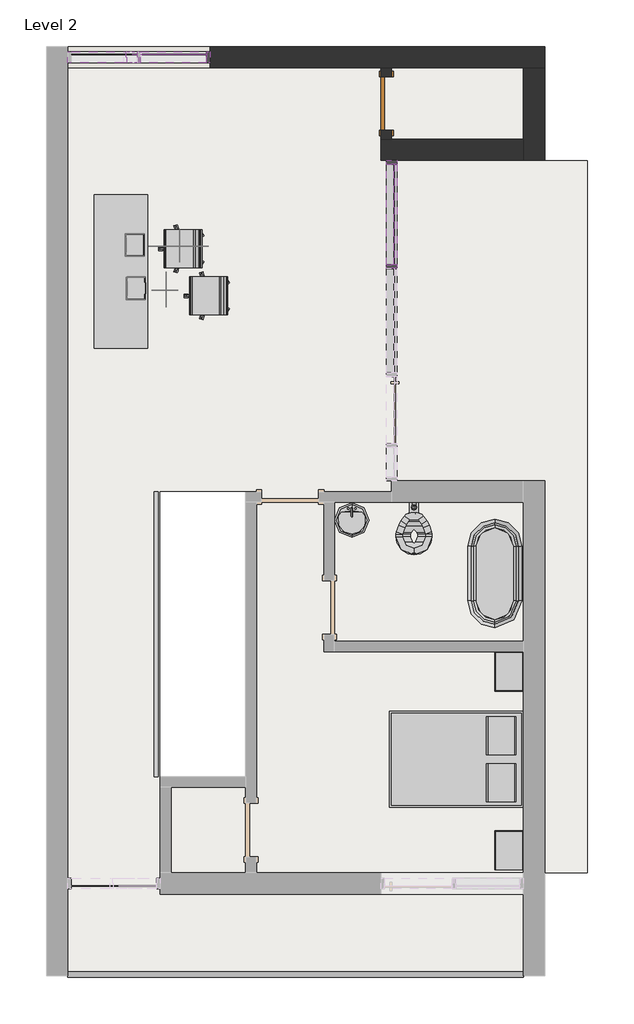
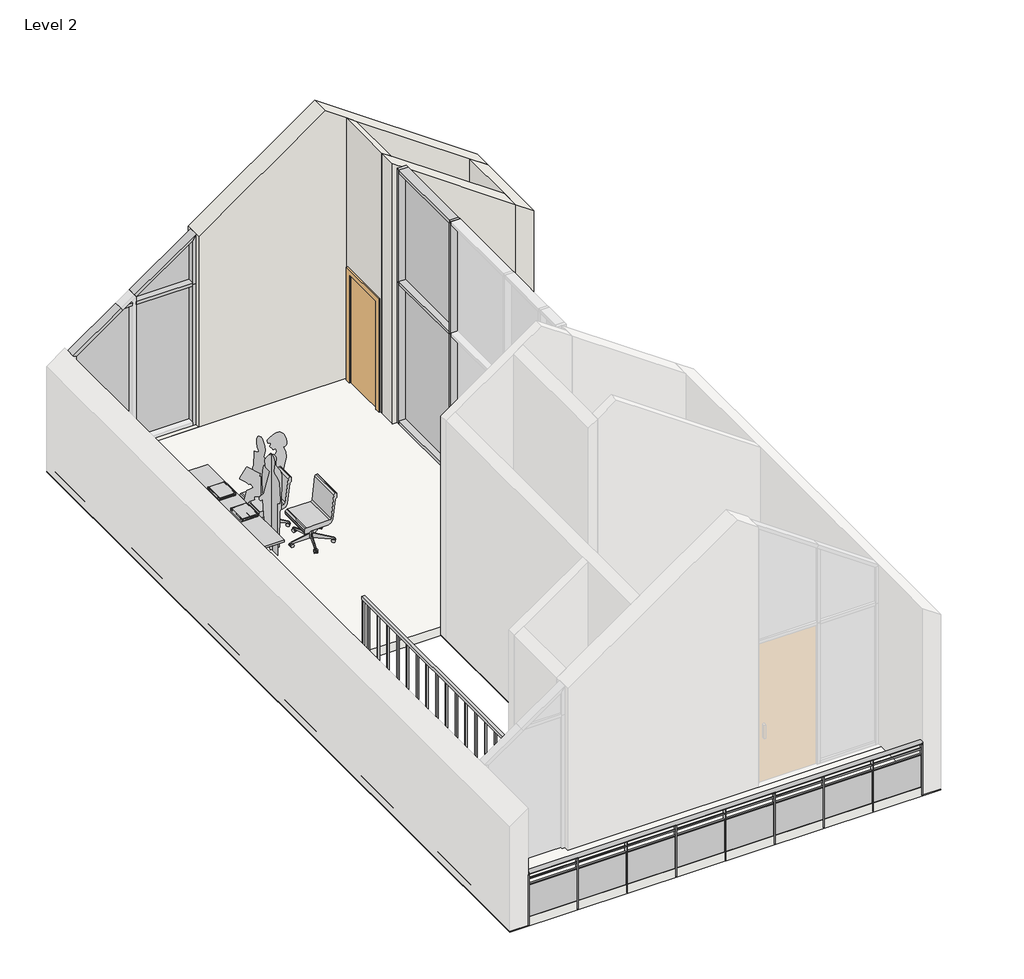
# One storey, part 2 of 2: 14 members, 6 furniture elements, 6 plates, 4 proxies, 4 walls, 3 flow terminals, 2 railings, 1 door, 1 slab.
"""IFC4 building model written with IfcOpenShell, lengths in millimetres."""

from ifc_helpers import new_model, si_unit, point, frame, origin, place, context, project, spatial, polyline, ellipse_curve, trimmed, outline, extrude, faceted_brep, transform, mapped, element, save
from ifc_brep_helpers import plane_surface, extruded_surface, advanced_brep
from components import entourage_d5009a78, m_rpc_female_e5f04239, m_rpc_male_90c61d85, m_door_single_flush_panel_double_acting_750_x_2000mm_e3d998e5, m_sink_vanity_round_482_x_482mm_721ec264, m_toilet_commercial_wall_3d_380mm_seat_height_4e8788ad, m_tub_free_standing_3d_760_x_1525mm_d9cb411c, m_bed_box_1346_x_1880mm_double_52b0093e, m_chair_task_m_chair_task_9903d5c1, m_furniture_system_standing_desk_rectangular_2150_x_750mm_604a6be1, m_furniture_system_storage_cabinet_2_drawer_400_x_550_x_4e0790d6, rectangular_mullion_50_x_150mm_116cff39, rectangular_mullion_50_x_150mm_695a1f45, rectangular_mullion_50_x_150mm_4a18de0c, rectangular_mullion_50_x_150mm_c59a77fc, rectangular_mullion_50_x_150mm_a16d5dba, rectangular_mullion_50_x_150mm_a2a5cdf7, rectangular_mullion_50_x_150mm_6c5cdad2, rectangular_mullion_50_x_150mm_cfe8f652, rectangular_mullion_50_x_150mm_e512abdd, rectangular_mullion_50_x_150mm_fd5e96fe, rectangular_mullion_50_x_150mm_6afb4452, rectangular_mullion_50_x_150mm_5b89cbb4, system_panel_glazed_60d66236, system_panel_glazed_9bec98e5, system_panel_glazed_53b80dfb, system_panel_glazed_816a57b3, system_panel_glazed_a9c2f29e, system_panel_glazed_28f5254f

model = new_model("IFC4")

# Units and contexts
model_context = context("Model", 3, world=origin())
ifc_project = project(units=[si_unit("LENGTHUNIT", "METRE", prefix="MILLI")], contexts=[model_context])

# Site, building, storey
site = spatial("IfcSite", under=ifc_project)
building = spatial("IfcBuilding", under=site)
storey = spatial("IfcBuildingStorey", under=building, Name="Level 2", Elevation=3200.0)

# Proxies
placement = place(None, origin())
entourage_shape = entourage_d5009a78(model_context)
element("IfcBuildingElementProxy", 1, Name="Entourage", at=placement, inside=storey, context=model_context, shape_type="MappedRepresentation", body=[
    mapped(entourage_shape, transform((-5449.0317552, 4088.4487917, 4083.3878119), x_axis=(0.0, -1.0, 0.0), y_axis=(1.0, 0.0, 0.0), z_axis=(0.0, 0.0, 1.0))),
])
element("IfcBuildingElementProxy", 2, Name="Entourage", at=placement, inside=storey, context=model_context, shape_type="MappedRepresentation", body=[
    mapped(entourage_shape, transform((-5464.0317552, 4697.034677, 4083.3878119), x_axis=(0.0, -1.0, 0.0), y_axis=(1.0, 0.0, 0.0), z_axis=(0.0, 0.0, 1.0))),
])
m_rpc_female_shape = m_rpc_female_e5f04239(model_context)
element("IfcBuildingElementProxy", 3, Name="M_RPC Female", ObjectType="M_RPC Female", at=placement, inside=storey, context=model_context, shape_type="MappedRepresentation", body=[
    mapped(m_rpc_female_shape, transform((-4960.0, 4682.9105508, 3333.3878119), x_axis=(0.0, 1.0, 0.0), y_axis=(-1.0, 0.0, 0.0), z_axis=(0.0, 0.0, 1.0))),
])
m_rpc_male_shape = m_rpc_male_90c61d85(model_context)
element("IfcBuildingElementProxy", 4, Name="M_RPC Male", ObjectType="M_RPC Male", at=placement, inside=storey, context=model_context, shape_type="MappedRepresentation", body=[
    mapped(m_rpc_male_shape, transform((-4985.7939615, 4076.4605844, 3200.0), x_axis=(0.0, 1.0, 0.0), y_axis=(-1.0, 0.0, 0.0), z_axis=(0.0, 0.0, 1.0))),
])

# Door
m_door_single_flush_panel_double_acting_750_x_2000mm_shape = m_door_single_flush_panel_double_acting_750_x_2000mm_e3d998e5(model_context)
element("IfcDoor", 5, ObjectType="M_Door-Single-Flush_Panel_Double-Acting : 750 x 2000mm", at=placement, inside=storey, context=model_context, shape_type="MappedRepresentation", body=[
    mapped(m_door_single_flush_panel_double_acting_750_x_2000mm_shape, transform((-1894.0317552, 6683.2522499, 3200.0), x_axis=(0.0, 1.0, 0.0), y_axis=(-1.0, 0.0, 0.0), z_axis=(0.0, 0.0, 1.0))),
])

# Flow terminals
m_sink_vanity_round_482_x_482mm_shape = m_sink_vanity_round_482_x_482mm_721ec264(model_context)
element("IfcFlowTerminal", 6, ObjectType="M_Sink Vanity-Round : 482 x 482mm", at=placement, inside=storey, context=model_context, shape_type="MappedRepresentation", body=[
    mapped(m_sink_vanity_round_482_x_482mm_shape, transform((-2475.6834958, 748.6049706, 3333.3878119), x_axis=(1.0, 0.0, 0.0), y_axis=(0.0, 1.0, 0.0), z_axis=(0.0, 0.0, 1.0))),
])
m_toilet_commercial_wall_3d_380mm_seat_height_shape = m_toilet_commercial_wall_3d_380mm_seat_height_4e8788ad(model_context)
element("IfcFlowTerminal", 7, ObjectType="M_Toilet-Commercial-Wall-3D : 380mm Seat Height", at=placement, inside=storey, context=model_context, shape_type="MappedRepresentation", body=[
    mapped(m_toilet_commercial_wall_3d_380mm_seat_height_shape, transform((-1100.1286014, 1233.2522499, 3200.0), x_axis=(-1.0, 0.0, 0.0), y_axis=(0.0, -1.0, 0.0), z_axis=(0.0, 0.0, 1.0))),
])
m_tub_free_standing_3d_760_x_1525mm_shape = m_tub_free_standing_3d_760_x_1525mm_d9cb411c(model_context)
element("IfcFlowTerminal", 8, ObjectType="M_Tub-Free Standing-3D : 760 x 1525mm", at=placement, inside=storey, context=model_context, shape_type="MappedRepresentation", body=[
    mapped(m_tub_free_standing_3d_760_x_1525mm_shape, transform((-369.0317552, 83.2522499, 3333.3878119), x_axis=(1.0, 0.0, 0.0), y_axis=(0.0, 1.0, 0.0), z_axis=(0.0, 0.0, 1.0))),
])

# Furniture
m_bed_box_1346_x_1880mm_double_shape = m_bed_box_1346_x_1880mm_double_52b0093e(model_context)
element("IfcFurniture", 9, ObjectType="M_Bed-Box : 1346 x 1880mm - Double", at=placement, inside=storey, context=model_context, shape_type="MappedRepresentation", body=[
    mapped(m_bed_box_1346_x_1880mm_double_shape, transform((-674.602247, -2184.5952911, 3333.3878119), x_axis=(0.0, -1.0, 0.0), y_axis=(1.0, 0.0, 0.0), z_axis=(0.0, 0.0, 1.0))),
])
m_chair_task_m_chair_task_shape = m_chair_task_m_chair_task_9903d5c1(model_context)
element("IfcFurniture", 10, ObjectType="M_Chair-Task : M_Chair-Task", at=placement, inside=storey, context=model_context, shape_type="MappedRepresentation", body=[
    mapped(m_chair_task_m_chair_task_shape, transform((-4730.0858536, 4502.2614302, 3333.3878119), x_axis=(0.0, 1.0, 0.0), y_axis=(-1.0, 0.0, 0.0), z_axis=(0.0, 0.0, 1.0))),
])
element("IfcFurniture", 11, ObjectType="M_Chair-Task : M_Chair-Task", at=placement, inside=storey, context=model_context, shape_type="MappedRepresentation", body=[
    mapped(m_chair_task_m_chair_task_shape, transform((-4370.0858536, 3842.2614302, 3333.3878119), x_axis=(0.0, 1.0, 0.0), y_axis=(-1.0, 0.0, 0.0), z_axis=(0.0, 0.0, 1.0))),
])
m_furniture_system_standing_desk_rectangular_2150_x_750mm_shape = m_furniture_system_standing_desk_rectangular_2150_x_750mm_604a6be1(model_context)
element("IfcFurniture", 12, ObjectType="M_Furniture_System-Standing_Desk-Rectangular : 2150 x 750mm", at=placement, inside=storey, context=model_context, shape_type="MappedRepresentation", body=[
    mapped(m_furniture_system_standing_desk_rectangular_2150_x_750mm_shape, transform((-6000.0, 3250.0, 3333.3878119), x_axis=(0.0, 1.0, 0.0), y_axis=(-1.0, 0.0, 0.0), z_axis=(0.0, 0.0, 1.0))),
])
m_furniture_system_storage_cabinet_2_drawer_400_x_550_x_shape = m_furniture_system_storage_cabinet_2_drawer_400_x_550_x_4e0790d6(model_context)
element("IfcFurniture", 13, ObjectType="M_Furniture_System-Storage-Cabinet-2_Drawer : 400 x 550 x 550mm", at=placement, inside=storey, context=model_context, shape_type="MappedRepresentation", body=[
    mapped(m_furniture_system_storage_cabinet_2_drawer_400_x_550_x_shape, transform((-169.0317552, -1566.7477501, 3333.3878119), x_axis=(1.0, 0.0, 0.0), y_axis=(0.0, 1.0, 0.0), z_axis=(0.0, 0.0, 1.0))),
])
element("IfcFurniture", 14, ObjectType="M_Furniture_System-Storage-Cabinet-2_Drawer : 400 x 550 x 550mm", at=placement, inside=storey, context=model_context, shape_type="MappedRepresentation", body=[
    mapped(m_furniture_system_storage_cabinet_2_drawer_400_x_550_x_shape, transform((-169.0317552, -3526.7477501, 3333.3878119), x_axis=(-1.0, 0.0, 0.0), y_axis=(0.0, -1.0, 0.0), z_axis=(0.0, 0.0, 1.0))),
])

# Members
rectangular_mullion_50_x_150mm_shape = rectangular_mullion_50_x_150mm_116cff39(model_context)
element("IfcMember", 15, ObjectType="Rectangular Mullion : 50 x 150mm", at=placement, inside=storey, context=model_context, shape_type="MappedRepresentation", body=[
    mapped(rectangular_mullion_50_x_150mm_shape, transform((-4419.0317552, 7333.2522499, 5758.3878119), x_axis=(0.0, 0.0, 1.0), y_axis=(0.0, -1.0, 0.0), z_axis=(1.0, 0.0, 0.0))),
])
rectangular_mullion_50_x_150mm_2_shape = rectangular_mullion_50_x_150mm_695a1f45(model_context)
element("IfcMember", 16, ObjectType="Rectangular Mullion : 50 x 150mm", at=placement, inside=storey, context=model_context, shape_type="MappedRepresentation", body=[
    mapped(rectangular_mullion_50_x_150mm_2_shape, transform((-1819.0317552, 5833.2522499, 3340.0348366), x_axis=(0.0, 0.0, -1.0), y_axis=(-1.0, 0.0, 0.0), z_axis=(0.0, 1.0, 0.0))),
])
rectangular_mullion_50_x_150mm_3_shape = rectangular_mullion_50_x_150mm_4a18de0c(model_context)
element("IfcMember", 17, ObjectType="Rectangular Mullion : 50 x 150mm", at=placement, inside=storey, context=model_context, shape_type="MappedRepresentation", body=[
    mapped(rectangular_mullion_50_x_150mm_3_shape, transform((-1819.0317552, 4366.5855831, 3340.0348366), x_axis=(0.0, 0.0, -1.0), y_axis=(-1.0, 0.0, 0.0), z_axis=(0.0, 1.0, 0.0))),
])
rectangular_mullion_50_x_150mm_4_shape = rectangular_mullion_50_x_150mm_c59a77fc(model_context)
element("IfcMember", 18, ObjectType="Rectangular Mullion : 50 x 150mm", at=placement, inside=storey, context=model_context, shape_type="MappedRepresentation", body=[
    mapped(rectangular_mullion_50_x_150mm_4_shape, transform((-1819.0317552, 4391.5855831, 3340.0348366), x_axis=(0.0, -1.0, 0.0), y_axis=(-1.0, 0.0, 0.0), z_axis=(0.0, 0.0, -1.0))),
])
element("IfcMember", 19, ObjectType="Rectangular Mullion : 50 x 150mm", at=placement, inside=storey, context=model_context, shape_type="MappedRepresentation", body=[
    mapped(rectangular_mullion_50_x_150mm_2_shape, transform((-1819.0317552, 4416.5855831, 7705.4462072), x_axis=(0.0, 0.0, 1.0), y_axis=(-1.0, 0.0, 0.0), z_axis=(0.0, -1.0, 0.0))),
])
rectangular_mullion_50_x_150mm_5_shape = rectangular_mullion_50_x_150mm_a16d5dba(model_context)
element("IfcMember", 20, ObjectType="Rectangular Mullion : 50 x 150mm", at=placement, inside=storey, context=model_context, shape_type="MappedRepresentation", body=[
    mapped(rectangular_mullion_50_x_150mm_5_shape, transform((-1819.0317552, 4391.5855831, 5765.0348366), x_axis=(0.0, -1.0, 0.0), y_axis=(-1.0, 0.0, 0.0), z_axis=(0.0, 0.0, -1.0))),
])
rectangular_mullion_50_x_150mm_6_shape = rectangular_mullion_50_x_150mm_a2a5cdf7(model_context)
element("IfcMember", 21, ObjectType="Rectangular Mullion : 50 x 150mm", at=placement, inside=storey, context=model_context, shape_type="MappedRepresentation", body=[
    mapped(rectangular_mullion_50_x_150mm_6_shape, transform((-1819.0317552, 4416.5855831, 5765.0348366), x_axis=(0.0, 0.0, 1.0), y_axis=(-1.0, 0.0, 0.0), z_axis=(0.0, -1.0, 0.0))),
])
rectangular_mullion_50_x_150mm_7_shape = rectangular_mullion_50_x_150mm_6c5cdad2(model_context)
element("IfcMember", 22, ObjectType="Rectangular Mullion : 50 x 150mm", at=placement, inside=storey, context=model_context, shape_type="MappedRepresentation", body=[
    mapped(rectangular_mullion_50_x_150mm_7_shape, transform((-4369.0317552, 7333.2522499, 6610.4773379), x_axis=(-0.5735764363510472, 0.0, 0.8191520442889909), y_axis=(0.0, -1.0, 0.0), z_axis=(0.8191520442889911, 0.0, 0.5735764363510473))),
])
rectangular_mullion_50_x_150mm_8_shape = rectangular_mullion_50_x_150mm_cfe8f652(model_context)
element("IfcMember", 23, ObjectType="Rectangular Mullion : 50 x 150mm", at=placement, inside=storey, context=model_context, shape_type="MappedRepresentation", body=[
    mapped(rectangular_mullion_50_x_150mm_8_shape, transform((-5585.9417133, 7333.2522499, 5758.3878119), x_axis=(-0.5735764363510475, 0.0, 0.8191520442889908), y_axis=(0.0, -1.0, 0.0), z_axis=(0.8191520442889908, 0.0, 0.5735764363510475))),
])
rectangular_mullion_50_x_150mm_9_shape = rectangular_mullion_50_x_150mm_e512abdd(model_context)
element("IfcMember", 24, ObjectType="Rectangular Mullion : 50 x 150mm", at=placement, inside=storey, context=model_context, shape_type="MappedRepresentation", body=[
    mapped(rectangular_mullion_50_x_150mm_9_shape, transform((-5394.0317552, 7333.2522499, 5758.3878119), x_axis=(0.0, 0.0, 1.0), y_axis=(0.0, -1.0, 0.0), z_axis=(1.0, 0.0, 0.0))),
])
rectangular_mullion_50_x_150mm_10_shape = rectangular_mullion_50_x_150mm_fd5e96fe(model_context)
element("IfcMember", 25, ObjectType="Rectangular Mullion : 50 x 150mm", at=placement, inside=storey, context=model_context, shape_type="MappedRepresentation", body=[
    mapped(rectangular_mullion_50_x_150mm_10_shape, transform((-4369.0317552, 7333.2522499, 3333.3878119), x_axis=(1.0, 0.0, 0.0), y_axis=(0.0, -1.0, 0.0), z_axis=(0.0, 0.0, -1.0))),
])
rectangular_mullion_50_x_150mm_11_shape = rectangular_mullion_50_x_150mm_6afb4452(model_context)
element("IfcMember", 26, ObjectType="Rectangular Mullion : 50 x 150mm", at=placement, inside=storey, context=model_context, shape_type="MappedRepresentation", body=[
    mapped(rectangular_mullion_50_x_150mm_11_shape, transform((-1819.0317552, 5883.2522499, 7705.4462072), x_axis=(0.0, 1.0, 0.0), y_axis=(-1.0, 0.0, 0.0), z_axis=(0.0, 0.0, 1.0))),
])
element("IfcMember", 27, ObjectType="Rectangular Mullion : 50 x 150mm", at=placement, inside=storey, context=model_context, shape_type="MappedRepresentation", body=[
    mapped(rectangular_mullion_50_x_150mm_10_shape, transform((-1819.0317552, 5883.2522499, 5765.0348366), x_axis=(0.0, 1.0, 0.0), y_axis=(-1.0, 0.0, 0.0), z_axis=(0.0, 0.0, 1.0))),
])
rectangular_mullion_50_x_150mm_12_shape = rectangular_mullion_50_x_150mm_5b89cbb4(model_context)
element("IfcMember", 28, ObjectType="Rectangular Mullion : 50 x 150mm", at=placement, inside=storey, context=model_context, shape_type="MappedRepresentation", body=[
    mapped(rectangular_mullion_50_x_150mm_12_shape, transform((-4369.0317552, 7333.2522499, 5758.3878119), x_axis=(1.0, 0.0, 0.0), y_axis=(0.0, -1.0, 0.0), z_axis=(0.0, 0.0, -1.0))),
])

# Plates
system_panel_glazed_shape = system_panel_glazed_60d66236(model_context)
element("IfcPlate", 29, ObjectType="System Panel : Glazed", at=placement, inside=storey, context=model_context, shape_type="MappedRepresentation", body=[
    mapped(system_panel_glazed_shape, transform((-5856.5317552, 7333.2522499, 3383.3878119), x_axis=(1.0, 0.0, 0.0), y_axis=(0.0, 1.0, 0.0), z_axis=(0.0, 0.0, 1.0))),
])
system_panel_glazed_2_shape = system_panel_glazed_9bec98e5(model_context)
element("IfcPlate", 30, ObjectType="System Panel : Glazed", at=placement, inside=storey, context=model_context, shape_type="MappedRepresentation", body=[
    mapped(system_panel_glazed_2_shape, transform((-4881.5317552, 7333.2522499, 3383.3878119), x_axis=(1.0, 0.0, 0.0), y_axis=(0.0, 1.0, 0.0), z_axis=(0.0, 0.0, 1.0))),
])
system_panel_glazed_3_shape = system_panel_glazed_53b80dfb(model_context)
element("IfcPlate", 31, ObjectType="System Panel : Glazed", at=placement, inside=storey, context=model_context, shape_type="MappedRepresentation", body=[
    mapped(system_panel_glazed_3_shape, transform((-1819.0317552, 5124.9189165, 3390.0348366), x_axis=(0.0, -1.0, 0.0), y_axis=(1.0, 0.0, 0.0), z_axis=(0.0, 0.0, 1.0))),
])
system_panel_glazed_4_shape = system_panel_glazed_816a57b3(model_context)
element("IfcPlate", 32, ObjectType="System Panel : Glazed", at=placement, inside=storey, context=model_context, shape_type="MappedRepresentation", body=[
    mapped(system_panel_glazed_4_shape, transform((-1819.0317552, 5124.9189165, 5790.0348366), x_axis=(0.0, -1.0, 0.0), y_axis=(1.0, 0.0, 0.0), z_axis=(0.0, 0.0, 1.0))),
])
system_panel_glazed_5_shape = system_panel_glazed_a9c2f29e(model_context)
element("IfcPlate", 33, ObjectType="System Panel : Glazed", at=placement, inside=storey, context=model_context, shape_type="MappedRepresentation", body=[
    mapped(system_panel_glazed_5_shape, transform((-5428.5487143, 7333.2522499, 5783.3878119), x_axis=(1.0, 0.0, 0.0), y_axis=(0.0, 1.0, 0.0), z_axis=(0.0, 0.0, 1.0))),
])
system_panel_glazed_6_shape = system_panel_glazed_28f5254f(model_context)
element("IfcPlate", 34, ObjectType="System Panel : Glazed", at=placement, inside=storey, context=model_context, shape_type="MappedRepresentation", body=[
    mapped(system_panel_glazed_6_shape, transform((-4881.5317552, 7333.2522499, 5783.3878119), x_axis=(1.0, 0.0, 0.0), y_axis=(0.0, 1.0, 0.0), z_axis=(0.0, 0.0, 1.0))),
])

# Railings
element("IfcRailing", 35, ObjectType="1100mm", at=placement, inside=storey, context=model_context, shape_type="SweptSolid", body=[
    extrude(outline(polyline([(-5104.0317552, -2766.7477501), (-5154.0317552, -2766.7477501), (-5154.0317552, 1233.2522499), (-5104.0317552, 1233.2522499), (-5104.0317552, -2766.7477501)])), frame((0.0, 0.0, 4250.0), z_axis=(0.0, 0.0, 1.0), x_axis=(1.0, 0.0, 0.0)), (0.0, 0.0, 1.0), 50.0),
    extrude(outline(polyline([(-5116.5317552, 1070.7522499), (-5141.5317552, 1070.7522499), (-5141.5317552, 1095.7522499), (-5116.5317552, 1095.7522499), (-5116.5317552, 1070.7522499)])), frame((0.0, 0.0, 3200.0), z_axis=(0.0, 0.0, 1.0), x_axis=(1.0, 0.0, 0.0)), (0.0, 0.0, 1.0), 1050.0),
    extrude(outline(polyline([(-5116.5317552, 795.7522499), (-5141.5317552, 795.7522499), (-5141.5317552, 820.7522499), (-5116.5317552, 820.7522499), (-5116.5317552, 795.7522499)])), frame((0.0, 0.0, 3200.0), z_axis=(0.0, 0.0, 1.0), x_axis=(1.0, 0.0, 0.0)), (0.0, 0.0, 1.0), 1050.0),
    extrude(outline(polyline([(-5116.5317552, 520.7522499), (-5141.5317552, 520.7522499), (-5141.5317552, 545.7522499), (-5116.5317552, 545.7522499), (-5116.5317552, 520.7522499)])), frame((0.0, 0.0, 3200.0), z_axis=(0.0, 0.0, 1.0), x_axis=(1.0, 0.0, 0.0)), (0.0, 0.0, 1.0), 1050.0),
    extrude(outline(polyline([(-5116.5317552, 245.7522499), (-5141.5317552, 245.7522499), (-5141.5317552, 270.7522499), (-5116.5317552, 270.7522499), (-5116.5317552, 245.7522499)])), frame((0.0, 0.0, 3200.0), z_axis=(0.0, 0.0, 1.0), x_axis=(1.0, 0.0, 0.0)), (0.0, 0.0, 1.0), 1050.0),
    extrude(outline(polyline([(-5116.5317552, -29.2477501), (-5141.5317552, -29.2477501), (-5141.5317552, -4.2477501), (-5116.5317552, -4.2477501), (-5116.5317552, -29.2477501)])), frame((0.0, 0.0, 3200.0), z_axis=(0.0, 0.0, 1.0), x_axis=(1.0, 0.0, 0.0)), (0.0, 0.0, 1.0), 1050.0),
    extrude(outline(polyline([(-5116.5317552, -304.2477501), (-5141.5317552, -304.2477501), (-5141.5317552, -279.2477501), (-5116.5317552, -279.2477501), (-5116.5317552, -304.2477501)])), frame((0.0, 0.0, 3200.0), z_axis=(0.0, 0.0, 1.0), x_axis=(1.0, 0.0, 0.0)), (0.0, 0.0, 1.0), 1050.0),
    extrude(outline(polyline([(-5116.5317552, -579.2477501), (-5141.5317552, -579.2477501), (-5141.5317552, -554.2477501), (-5116.5317552, -554.2477501), (-5116.5317552, -579.2477501)])), frame((0.0, 0.0, 3200.0), z_axis=(0.0, 0.0, 1.0), x_axis=(1.0, 0.0, 0.0)), (0.0, 0.0, 1.0), 1050.0),
    extrude(outline(polyline([(-5116.5317552, -854.2477501), (-5141.5317552, -854.2477501), (-5141.5317552, -829.2477501), (-5116.5317552, -829.2477501), (-5116.5317552, -854.2477501)])), frame((0.0, 0.0, 3200.0), z_axis=(0.0, 0.0, 1.0), x_axis=(1.0, 0.0, 0.0)), (0.0, 0.0, 1.0), 1050.0),
    extrude(outline(polyline([(-5116.5317552, -1129.2477501), (-5141.5317552, -1129.2477501), (-5141.5317552, -1104.2477501), (-5116.5317552, -1104.2477501), (-5116.5317552, -1129.2477501)])), frame((0.0, 0.0, 3200.0), z_axis=(0.0, 0.0, 1.0), x_axis=(1.0, 0.0, 0.0)), (0.0, 0.0, 1.0), 1050.0),
    extrude(outline(polyline([(-5116.5317552, -1404.2477501), (-5141.5317552, -1404.2477501), (-5141.5317552, -1379.2477501), (-5116.5317552, -1379.2477501), (-5116.5317552, -1404.2477501)])), frame((0.0, 0.0, 3200.0), z_axis=(0.0, 0.0, 1.0), x_axis=(1.0, 0.0, 0.0)), (0.0, 0.0, 1.0), 1050.0),
    extrude(outline(polyline([(-5116.5317552, -1679.2477501), (-5141.5317552, -1679.2477501), (-5141.5317552, -1654.2477501), (-5116.5317552, -1654.2477501), (-5116.5317552, -1679.2477501)])), frame((0.0, 0.0, 3200.0), z_axis=(0.0, 0.0, 1.0), x_axis=(1.0, 0.0, 0.0)), (0.0, 0.0, 1.0), 1050.0),
    extrude(outline(polyline([(-5116.5317552, -1954.2477501), (-5141.5317552, -1954.2477501), (-5141.5317552, -1929.2477501), (-5116.5317552, -1929.2477501), (-5116.5317552, -1954.2477501)])), frame((0.0, 0.0, 3200.0), z_axis=(0.0, 0.0, 1.0), x_axis=(1.0, 0.0, 0.0)), (0.0, 0.0, 1.0), 1050.0),
    extrude(outline(polyline([(-5116.5317552, -2229.2477501), (-5141.5317552, -2229.2477501), (-5141.5317552, -2204.2477501), (-5116.5317552, -2204.2477501), (-5116.5317552, -2229.2477501)])), frame((0.0, 0.0, 3200.0), z_axis=(0.0, 0.0, 1.0), x_axis=(1.0, 0.0, 0.0)), (0.0, 0.0, 1.0), 1050.0),
    extrude(outline(polyline([(-5116.5317552, -2504.2477501), (-5141.5317552, -2504.2477501), (-5141.5317552, -2479.2477501), (-5116.5317552, -2479.2477501), (-5116.5317552, -2504.2477501)])), frame((0.0, 0.0, 3200.0), z_axis=(0.0, 0.0, 1.0), x_axis=(1.0, 0.0, 0.0)), (0.0, 0.0, 1.0), 1050.0),
    extrude(outline(polyline([(-5116.5317552, 1208.2522499), (-5141.5317552, 1208.2522499), (-5141.5317552, 1233.2522499), (-5116.5317552, 1233.2522499), (-5116.5317552, 1208.2522499)])), frame((0.0, 0.0, 3200.0), z_axis=(0.0, 0.0, 1.0), x_axis=(1.0, 0.0, 0.0)), (0.0, 0.0, 1.0), 1050.0),
    extrude(outline(polyline([(-5116.5317552, -2766.7477501), (-5141.5317552, -2766.7477501), (-5141.5317552, -2741.7477501), (-5116.5317552, -2741.7477501), (-5116.5317552, -2766.7477501)])), frame((0.0, 0.0, 3200.0), z_axis=(0.0, 0.0, 1.0), x_axis=(1.0, 0.0, 0.0)), (0.0, 0.0, 1.0), 1050.0),
])
element("IfcRailing", 36, ObjectType="Glass Panel - Bottom Fill", at=placement, inside=storey, context=model_context, shape_type="SolidModel", body=[
    advanced_brep(
    [(-6369.0317552, -5507.356985, 4100.0), (-6369.0317552, -5587.356985, 4100.0), (30.9682448, -5507.356985, 4100.0), (30.9682448, -5587.356985, 4100.0)],
    [
        (0, 1, ellipse_curve(frame((-6369.0317552, -5547.356985, 4100.0), z_axis=(-1.0, 0.0, 0.0), x_axis=(0.0, -1.0, 0.0)), 40.0, 30.0)),
        (1, 0, ellipse_curve(frame((-6369.0317552, -5547.356985, 4100.0), z_axis=(-1.0, 0.0, 0.0), x_axis=(0.0, -1.0, 0.0)), 40.0, 30.0)),
        (2, 3, ellipse_curve(frame((30.9682448, -5547.356985, 4100.0), z_axis=(1.0, 0.0, 0.0), x_axis=(0.0, -1.0, 0.0)), 40.0, 30.0)),
        (3, 2, ellipse_curve(frame((30.9682448, -5547.356985, 4100.0), z_axis=(1.0, 0.0, 0.0), x_axis=(0.0, -1.0, 0.0)), 40.0, 30.0)),
        (0, 2),
        (3, 1),
    ],
    [
        plane_surface(frame((-6369.0317552, -5547.356985, 4100.0), z_axis=(-1.0, 0.0, 0.0), x_axis=(0.0, 1.0, 0.0))),
        plane_surface(frame((30.9682448, -5547.356985, 4100.0), z_axis=(1.0, 0.0, 0.0), x_axis=(0.0, 1.0, 0.0))),
        extruded_surface(trimmed(ellipse_curve(frame((30.9682448, -5547.356985, 4100.0), z_axis=(-1.0, 0.0, 0.0), x_axis=(0.0, -1.0, 0.0)), 40.0, 30.0), [point((30.9682448, -5507.356985, 4100.0))], [point((30.9682448, -5587.356985, 4100.0))], True, "CARTESIAN"), (-6400.0, 0.0, 0.0), 6400.0),
        extruded_surface(trimmed(ellipse_curve(frame((30.9682448, -5547.356985, 4100.0), z_axis=(-1.0, 0.0, 0.0), x_axis=(0.0, -1.0, 0.0)), 40.0, 30.0), [point((30.9682448, -5587.356985, 4100.0))], [point((30.9682448, -5507.356985, 4100.0))], True, "CARTESIAN"), (-6400.0, 0.0, 0.0), 6400.0),
    ],
    [
        (0, [[1, 2]]),
        (1, [[3, 4]]),
        (2, [[-1, 5, -4, 6]]),
        (3, [[-2, -6, -3, -5]]),
    ],
),
    extrude(outline(polyline([(-6369.0317552, -5556.7477501), (-6369.0317552, -5536.7477501), (30.9682448, -5536.7477501), (30.9682448, -5556.7477501), (-6369.0317552, -5556.7477501)])), frame((0.0, 0.0, 3980.0), z_axis=(0.0, 0.0, 1.0), x_axis=(1.0, 0.0, 0.0)), (0.0, 0.0, 1.0), 20.0),
    extrude(outline(polyline([(-6369.0317552, -5556.7477501), (-6369.0317552, -5536.7477501), (30.9682448, -5536.7477501), (30.9682448, -5556.7477501), (-6369.0317552, -5556.7477501)])), frame((0.0, 0.0, 3880.0), z_axis=(0.0, 0.0, 1.0), x_axis=(1.0, 0.0, 0.0)), (0.0, 0.0, 1.0), 20.0),
    extrude(outline(polyline([(-769.0317552, -5548.4725602), (30.9682448, -5548.4725602), (30.9682448, -5553.4725602), (-769.0317552, -5553.4725602), (-769.0317552, -5548.4725602)])), frame((0.0, 0.0, 3300.0), z_axis=(0.0, 0.0, 1.0), x_axis=(1.0, 0.0, 0.0)), (0.0, 0.0, 1.0), 580.0),
    extrude(outline(polyline([(-775.0317552, -5521.7477501), (-763.0317552, -5521.7477501), (-763.0317552, -5571.7477501), (-775.0317552, -5571.7477501), (-775.0317552, -5521.7477501)])), frame((0.0, 0.0, 3200.0), z_axis=(0.0, 0.0, 1.0), x_axis=(1.0, 0.0, 0.0)), (0.0, 0.0, 1.0), 870.0),
    extrude(outline(polyline([(-1569.0317552, -5548.4725602), (-769.0317552, -5548.4725602), (-769.0317552, -5553.4725602), (-1569.0317552, -5553.4725602), (-1569.0317552, -5548.4725602)])), frame((0.0, 0.0, 3300.0), z_axis=(0.0, 0.0, 1.0), x_axis=(1.0, 0.0, 0.0)), (0.0, 0.0, 1.0), 580.0),
    extrude(outline(polyline([(-1575.0317552, -5521.7477501), (-1563.0317552, -5521.7477501), (-1563.0317552, -5571.7477501), (-1575.0317552, -5571.7477501), (-1575.0317552, -5521.7477501)])), frame((0.0, 0.0, 3200.0), z_axis=(0.0, 0.0, 1.0), x_axis=(1.0, 0.0, 0.0)), (0.0, 0.0, 1.0), 870.0),
    extrude(outline(polyline([(-2369.0317552, -5548.4725602), (-1569.0317552, -5548.4725602), (-1569.0317552, -5553.4725602), (-2369.0317552, -5553.4725602), (-2369.0317552, -5548.4725602)])), frame((0.0, 0.0, 3300.0), z_axis=(0.0, 0.0, 1.0), x_axis=(1.0, 0.0, 0.0)), (0.0, 0.0, 1.0), 580.0),
    extrude(outline(polyline([(-2375.0317552, -5521.7477501), (-2363.0317552, -5521.7477501), (-2363.0317552, -5571.7477501), (-2375.0317552, -5571.7477501), (-2375.0317552, -5521.7477501)])), frame((0.0, 0.0, 3200.0), z_axis=(0.0, 0.0, 1.0), x_axis=(1.0, 0.0, 0.0)), (0.0, 0.0, 1.0), 870.0),
    extrude(outline(polyline([(-3169.0317552, -5548.4725602), (-2369.0317552, -5548.4725602), (-2369.0317552, -5553.4725602), (-3169.0317552, -5553.4725602), (-3169.0317552, -5548.4725602)])), frame((0.0, 0.0, 3300.0), z_axis=(0.0, 0.0, 1.0), x_axis=(1.0, 0.0, 0.0)), (0.0, 0.0, 1.0), 580.0),
    extrude(outline(polyline([(-3175.0317552, -5521.7477501), (-3163.0317552, -5521.7477501), (-3163.0317552, -5571.7477501), (-3175.0317552, -5571.7477501), (-3175.0317552, -5521.7477501)])), frame((0.0, 0.0, 3200.0), z_axis=(0.0, 0.0, 1.0), x_axis=(1.0, 0.0, 0.0)), (0.0, 0.0, 1.0), 870.0),
    extrude(outline(polyline([(-3969.0317552, -5548.4725602), (-3169.0317552, -5548.4725602), (-3169.0317552, -5553.4725602), (-3969.0317552, -5553.4725602), (-3969.0317552, -5548.4725602)])), frame((0.0, 0.0, 3300.0), z_axis=(0.0, 0.0, 1.0), x_axis=(1.0, 0.0, 0.0)), (0.0, 0.0, 1.0), 580.0),
    extrude(outline(polyline([(-3975.0317552, -5521.7477501), (-3963.0317552, -5521.7477501), (-3963.0317552, -5571.7477501), (-3975.0317552, -5571.7477501), (-3975.0317552, -5521.7477501)])), frame((0.0, 0.0, 3200.0), z_axis=(0.0, 0.0, 1.0), x_axis=(1.0, 0.0, 0.0)), (0.0, 0.0, 1.0), 870.0),
    extrude(outline(polyline([(-4769.0317552, -5548.4725602), (-3969.0317552, -5548.4725602), (-3969.0317552, -5553.4725602), (-4769.0317552, -5553.4725602), (-4769.0317552, -5548.4725602)])), frame((0.0, 0.0, 3300.0), z_axis=(0.0, 0.0, 1.0), x_axis=(1.0, 0.0, 0.0)), (0.0, 0.0, 1.0), 580.0),
    extrude(outline(polyline([(-4775.0317552, -5521.7477501), (-4763.0317552, -5521.7477501), (-4763.0317552, -5571.7477501), (-4775.0317552, -5571.7477501), (-4775.0317552, -5521.7477501)])), frame((0.0, 0.0, 3200.0), z_axis=(0.0, 0.0, 1.0), x_axis=(1.0, 0.0, 0.0)), (0.0, 0.0, 1.0), 870.0),
    extrude(outline(polyline([(-5569.0317552, -5548.4725602), (-4769.0317552, -5548.4725602), (-4769.0317552, -5553.4725602), (-5569.0317552, -5553.4725602), (-5569.0317552, -5548.4725602)])), frame((0.0, 0.0, 3300.0), z_axis=(0.0, 0.0, 1.0), x_axis=(1.0, 0.0, 0.0)), (0.0, 0.0, 1.0), 580.0),
    extrude(outline(polyline([(-5575.0317552, -5521.7477501), (-5563.0317552, -5521.7477501), (-5563.0317552, -5571.7477501), (-5575.0317552, -5571.7477501), (-5575.0317552, -5521.7477501)])), frame((0.0, 0.0, 3200.0), z_axis=(0.0, 0.0, 1.0), x_axis=(1.0, 0.0, 0.0)), (0.0, 0.0, 1.0), 870.0),
    extrude(outline(polyline([(-6369.0317552, -5548.4725602), (-5569.0317552, -5548.4725602), (-5569.0317552, -5553.4725602), (-6369.0317552, -5553.4725602), (-6369.0317552, -5548.4725602)])), frame((0.0, 0.0, 3300.0), z_axis=(0.0, 0.0, 1.0), x_axis=(1.0, 0.0, 0.0)), (0.0, 0.0, 1.0), 580.0),
    extrude(outline(polyline([(22.9682448, -5521.7477501), (34.9682448, -5521.7477501), (34.9682448, -5571.7477501), (22.9682448, -5571.7477501), (22.9682448, -5521.7477501)])), frame((0.0, 0.0, 3200.0), z_axis=(0.0, 0.0, 1.0), x_axis=(1.0, 0.0, 0.0)), (0.0, 0.0, 1.0), 870.0),
    extrude(outline(polyline([(-6373.0317552, -5521.7477501), (-6361.0317552, -5521.7477501), (-6361.0317552, -5571.7477501), (-6373.0317552, -5571.7477501), (-6373.0317552, -5521.7477501)])), frame((0.0, 0.0, 3200.0), z_axis=(0.0, 0.0, 1.0), x_axis=(1.0, 0.0, 0.0)), (0.0, 0.0, 1.0), 870.0),
])

# Slab
element("IfcSlab", 37, ObjectType="Generic 150mm", at=placement, inside=storey, context=model_context, shape_type="SweptSolid", body=[
    extrude(outline(polyline([(-6669.0317552, 7483.2522499), (330.9682448, 7483.2522499), (330.9682448, 5883.2522499), (930.9682448, 5883.2522499), (930.9682448, -4116.7477501), (330.9682448, -4116.7477501), (330.9682448, -5566.7477501), (-6669.0317552, -5566.7477501), (-6669.0317552, 7483.2522499)]), holes=[polyline([(-3869.0317552, 1233.2522499), (-5069.0317552, 1233.2522499), (-5069.0317552, -2766.7477501), (-3869.0317552, -2766.7477501), (-3869.0317552, 1233.2522499)])]), frame((0.0, 0.0, 3183.3878119), z_axis=(0.0, 0.0, 1.0), x_axis=(1.0, 0.0, 0.0)), (0.0, 0.0, 1.0), 150.0),
])

# Walls
element("IfcWall", 38, ObjectType="Generic - 300mm", at=placement, inside=storey, context=model_context, shape_type="Brep", body=[
    faceted_brep([(330.9682448, 7483.2522499, 3200.0), (-6369.0317552, 7483.2522499, 3200.0), (-6369.0317552, 7483.2522499, 3333.3878119), (-4369.0317552, 7483.2522499, 3333.3878119), (-4369.0317552, 7483.2522499, 6610.4773379), (-2312.1429511, 7483.2522499, 8050.7263837), (330.9682448, 7483.2522499, 6200.0), (-6369.0317552, 7183.2522499, 3200.0), (-1969.0317552, 7183.2522499, 3200.0), (-1819.0317552, 7183.2522499, 3200.0), (30.9682448, 7183.2522499, 3200.0), (330.9682448, 7183.2522499, 3200.0), (330.9682448, 7183.2522499, 6200.0), (30.9682448, 7183.2522499, 6410.0622615), (-1819.0317552, 7183.2522499, 7705.4462072), (-1969.0317552, 7183.2522499, 7810.4773379), (-2312.1429511, 7183.2522499, 8050.7263837), (-4369.0317552, 7183.2522499, 6610.4773379), (-4369.0317552, 7183.2522499, 3333.3878119), (-6369.0317552, 7183.2522499, 3333.3878119)], [[[0, 1, 2, 3, 4, 5, 6]], [[7, 8, 9, 10, 11, 12, 13, 14, 15, 16, 17, 18, 19]], [[1, 0, 11, 10, 9, 8, 7]], [[0, 6, 12, 11]], [[1, 7, 19, 2]], [[3, 18, 17, 4]], [[18, 3, 2, 19]], [[12, 6, 5, 16, 15, 14, 13]], [[16, 5, 4, 17]]]),
])
element("IfcWall", 39, ObjectType="Generic - 300mm", at=placement, inside=storey, context=model_context, shape_type="Brep", body=[
    faceted_brep([(30.9682448, 6183.2522499, 6410.0622615), (30.9682448, 6183.2522499, 3200.0), (-1819.0317552, 6183.2522499, 3200.0), (-1969.0317552, 6183.2522499, 3200.0), (-1969.0317552, 6183.2522499, 7810.4773379), (-1819.0317552, 6183.2522499, 7705.4462072), (30.9682448, 5883.2522499, 3200.0), (30.9682448, 5883.2522499, 4100.0), (30.9682448, 5883.2522499, 6410.0622615), (-1744.0317552, 5883.2522499, 7652.9306418), (-1969.0317552, 5883.2522499, 7810.4773379), (-1969.0317552, 5883.2522499, 3200.0)], [[[0, 1, 2, 3, 4, 5]], [[6, 7, 8, 9, 10, 11]], [[3, 2, 1, 6, 11]], [[4, 3, 11, 10]], [[0, 8, 7, 6, 1]], [[0, 5, 4, 10, 9, 8]]]),
])
element("IfcWall", 40, ObjectType="Generic - 300mm", at=placement, inside=storey, context=model_context, shape_type="Brep", body=[
    faceted_brep([(330.9682448, 6183.2522499, 4100.0), (330.9682448, 6183.2522499, 3200.0), (330.9682448, 7183.2522499, 3200.0), (330.9682448, 7183.2522499, 6200.0), (330.9682448, 5883.2522499, 6200.0), (330.9682448, 5883.2522499, 4100.0), (30.9682448, 6183.2522499, 3200.0), (30.9682448, 6183.2522499, 4100.0), (30.9682448, 5883.2522499, 4100.0), (30.9682448, 5883.2522499, 6410.0622615), (30.9682448, 6183.2522499, 6410.0622615), (30.9682448, 7183.2522499, 6410.0622615), (30.9682448, 7183.2522499, 3200.0)], [[[0, 1, 2, 3, 4, 5]], [[6, 7, 8, 9, 10, 11, 12]], [[2, 1, 6, 12]], [[3, 2, 12, 11]], [[5, 8, 7, 0]], [[0, 7, 6, 1]], [[5, 4, 9, 8]], [[4, 3, 11, 10, 9]]]),
])
element("IfcWall", 41, ObjectType="small inner wall 150mm", at=placement, inside=storey, context=model_context, shape_type="Brep", body=[
    faceted_brep([(-1819.0317552, 6183.2522499, 7705.4462072), (-1819.0317552, 6183.2522499, 3200.0), (-1819.0317552, 6308.2522499, 3200.0), (-1819.0317552, 6308.2522499, 5200.0), (-1819.0317552, 7058.2522499, 5200.0), (-1819.0317552, 7058.2522499, 3200.0), (-1819.0317552, 7183.2522499, 3200.0), (-1819.0317552, 7183.2522499, 7705.4462072), (-1969.0317552, 6183.2522499, 3200.0), (-1969.0317552, 6183.2522499, 7810.4773379), (-1969.0317552, 7183.2522499, 7810.4773379), (-1969.0317552, 7183.2522499, 3200.0), (-1969.0317552, 7058.2522499, 3200.0), (-1969.0317552, 7058.2522499, 5200.0), (-1969.0317552, 6308.2522499, 5200.0), (-1969.0317552, 6308.2522499, 3200.0)], [[[0, 1, 2, 3, 4, 5, 6, 7]], [[8, 9, 10, 11, 12, 13, 14, 15]], [[1, 8, 15, 2]], [[11, 6, 5, 12]], [[1, 0, 9, 8]], [[7, 6, 11, 10]], [[4, 13, 12, 5]], [[14, 3, 2, 15]], [[0, 7, 10, 9]], [[3, 14, 13, 4]]]),
])

save(model, "model.ifc")

# Revit data of these elements
# Type
#   built-in parameter 1005198 = "{2, 15},{39, RPC-16-N04H-AQSP-D1N4-43SU-6GKQ-C3KU-1C},{1, 0},{1, 0},{2, 41},{1, 8},{5, Color},{1, 0},{1, 0},{3, 0.8},{3, 0.8},{3, 0.8},{1, 8},{7, BBoxMin},{1, 0},{1, 0},{1, 0},{1, 0},{1, 0},{1, 8},{7, BBoxMax},{1, 0},{1, 0},{1, 0},{1, 0},{1, 0},{2, 11},{9, RPCTypeId},{1, 0},{1, 0},{39, RPC-16-N04H-AQSP-D1N4-43SU-6GKQ-C3KU-1C},{1, 6},{14, RPCPlantHeight},{1, 0},{1, 0},{7, 2.28517},{2, 11},{7, keyword},{1, 0},{1, 0},{31, :Geometry:RPC:Notebook Computer},{2, 11},{8, category},{1, 0},{1, 0},{15, :Office Clutter},{2, 11},{12, LocalizedUID},{1, 0},{1, 0},{17, Notebook Computer},{2, 14},{6, Height},{1, 0},{1, 0},{7, 2.28517},{1, 2},{16, Cast Reflections},{1, 0},{1, 0},{1, 0},{1, 4},{4, Open},{1, 0},{1, 0},{4, -106},{1, 2},{5, Power},{1, 0},{1, 0},{1, 1},{2, 11},{14, Screen Preview},{1, 0},{1, 0},{70, __RPC:/object data/textures/object/Top/TopScreen/textures/on/rgb/0/0/0},{2, 11},{16, i_Screen Preview},{1, 0},{1, 0},{0, },{1, 2},{13, Custom Screen},{1, 0},{1, 0},{1, 0},{2, 11},{16, Screen File Name},{1, 0},{1, 0},{0, },{2, 11},{20, AdvancedUIDefinition},{1, 0},{1, 0},{0, },{2, 11},{10, AssetLibID},{1, 0},{1, 0},{36, 4D3F6E72-3F99-4203-98E9-AF80B3C7A7A4},{2, 11},{10, BaseSchema},{1, 0},{1, 0},{9, RPCSchema},{2, 11},{12, ExchangeGUID},{1, 0},{1, 0},{0, },{1, 2},{6, Hidden},{1, 0},{1, 0},{1, 0},{1, 4},{11, RPCCategory},{1, 0},{1, 0},{1, 0},{2, 11},{8, RPCImage},{1, 0},{1, 0},{0, },{1, 4},{13, SchemaVersion},{1, 0},{1, 0},{1, 4},{2, 11},{12, UIDefinition},{1, 0},{1, 0},{0, },{2, 11},{6, UIName},{1, 0},{1, 0},{39, RPC-16-N04H-AQSP-D1N4-43SU-6GKQ-C3KU-1C},{2, 11},{11, VersionGUID},{1, 0},{1, 0},{9, RPCSchema},{2, 11},{9, assettype},{1, 0},{1, 0},{11, RPCGeometry},{2, 11},{11, description},{1, 0},{1, 0},{0, },{2, 11},{9, localname},{1, 0},{1, 0},{3, RPC},{2, 11},{9, localtype},{1, 0},{1, 0},{3, RPC},{1, 4},{8, revision},{1, 0},{1, 0},{1, 1},{2, 11},{9, thumbnail},{1, 0},{1, 0},{0, },{1, 4},{7, version},{1, 0},{1, 0},{1, 1},{1, 2},{20, RPC_Cast Reflections},{1, 0},{1, 0},{1, 1},{1, 4},{8, RPC_Open},{1, 0},{1, 0},{4, -106},{1, 2},{9, RPC_Power},{1, 0},{1, 0},{1, 1},{2, 11},{18, RPC_Screen Preview},{1, 0},{1, 0},{70, __RPC:/object data/textures/object/Top/TopScreen/textures/on/rgb/0/0/0},{2, 11},{20, RPC_i_Screen Preview},{1, 0},{1, 0},{0, },{1, 2},{17, RPC_Custom Screen},{1, 0},{1, 0},{1, 0},{2, 11},{20, RPC_Screen File Name},{1, 0},{1, 0},{0, },{21, assetlibrary_base.fbx},{1, 5},"
#   built-in parameter 1005195 = "RPC-16-N04H-AQSP-D1N4-43SU-6GKQ-C3KU-1C"
#   Height = 0
# Type "M_RPC Female"
#   built-in parameter 1005195 = "RPC-8-FXA2-QQQ0-UGV2-6"
#   Height = 0
# Type "M_RPC Male"
#   built-in parameter 1005195 = "RPC-8-G1AE-S4G0-CKUK-A"
#   Height = 0
# Type "M_Door-Single-Flush_Panel_Double-Acting : 750 x 2000mm"
#   Type Mark = "45"
#   Construction Type Id = "DOOR"
#   Assembly Code = "C1020300"
#   Analytic Construction = "Wooden"
#   Thickness = 50 mm
#   Thermal Resistance (R) = 0.455703 (m²·K)/W
#   Swing Angle [instance default] = 90.00°
#   Heat Transfer Coefficient (U) = 2.19465 W/(m²·K)
#   Height = 2000 mm
#   Trim Projection Ext. = 25 mm
#   Trim Projection Int. = 25 mm
#   Trim Width Ext. = 80 mm
#   Trim Width Int. = 80 mm
#   Width = 750 mm
#   Define Thermal Properties by = 1
#   Trim Material = Paint - Sienna
#   Panel Material = Wood - Birch - Solid Stained Light Low Gloss
#   Visual Light Transmittance = 0
#   Solar Heat Gain Coefficient = 0
#   Function = (empty or 0)
#   Wall Closure = (empty or 0)
# Type "M_Sink Vanity-Round : 482 x 482mm"
#   Top Of Counter [instance default] = 750 mm
#   Basin Material = Porcelain, Linen
#   Fixture Material = Steel, Polished
#   Default Elevation = 0
# Type "M_Toilet-Commercial-Wall-3D : 380mm Seat Height"
#   Mounting Height = 380 mm
#   Piping Material = Steel, Polished
#   Bowl Material = Porcelain, Ivory
#   Seat Material = Laminate, Ivory, Matte
#   Default Elevation = 0
# Type "M_Tub-Free Standing-3D : 760 x 1525mm"
#   Height = 460 mm
#   Length = 1525 mm
#   Width = 760 mm
#   Tub Material = Porcelain, Ivory
#   Default Elevation = 0
# Type "M_Bed-Box : 1346 x 1880mm - Double"
#   Length = 1880 mm
#   Width = 1346 mm
#   Frame Material = Birch
#   Mattress Material = Linen, White
#   Default Elevation = 0
# Type "M_Chair-Task : M_Chair-Task"
#   Base Material = Plastic, Opaque Black
#   Caster Material = Plastic, Opaque Black
#   Seat/Back Material = Textile - Slate Blue
#   Default Elevation = 0
# Type "M_Furniture_System-Standing_Desk-Rectangular : 2150 x 750mm"
#   Type Comments = "2150 x 750mm Rectangular Standing Desk"
#   Thickness = 30 mm
#   Width = 2150 mm
#   Height [instance default] = 750 mm
#   H [instance default] = 755 mm
#   Foot Height [instance default] = 720 mm
#   Depth = 750 mm
#   Work Surface Material [instance default] = Plastic Laminate - White Oak
#   Foot Material [instance default] = Metal - Paint Linen
#   Edge Material [instance default] = Plastic Laminate - Beige - Light - Smooth
#   Model = ""
#   Manufacturer = ""
#   Description = (empty or 0)
#   Default Elevation = 0
# Type "M_Furniture_System-Storage-Cabinet-2_Drawer : 400 x 550 x 550mm"
#   Type Comments = "400 x 550 x 550mm Double Drawer Cabinet"
#   Width = 400 mm
#   Height = 550 mm
#   Depth = 550 mm
#   Show Solid [instance default] = yes
#   Show Dashed [instance default] = no
#   Seat Visible [instance default] = yes
#   Drawer Material [instance default] = Metal - Paint - Beige
#   Cabinet Material [instance default] = Metal - Paint - Beige
#   Model = ""
#   Manufacturer = ""
#   Keynote = ""
#   Description = (empty or 0)
#   Default Elevation = 0
# Type "Rectangular Mullion : 50 x 150mm"
#   built-in parameter 1007304 = 0.492126 (stored number, unit not read)
#   built-in parameter 1007301 = 0.082021 (stored number, unit not read)
#   built-in parameter 1007300 = 0.082021 (stored number, unit not read)
# Type "System Panel : Glazed"
#   Construction Type Id = "GSP4R"
#   Analytic Construction = "1/8 in Pilkington single glazing"
#   Visual Light Transmittance = 0.9
#   Solar Heat Gain Coefficient = 0.86
#   Heat Transfer Coefficient (U) = 6.7069 W/(m²·K)
#   Define Thermal Properties by = 1
# Type "1100mm"
#   built-in parameter 1008612 = 0.019685 (stored number, unit not read)
#   built-in parameter 1008611 = 0.019685 (stored number, unit not read)
#   built-in parameter 1008609 = 0.902231 (stored number, unit not read)
#   built-in parameter 1008604 = 0.19685 (stored number, unit not read)
#   built-in parameter 1008603 = 0.164042 (stored number, unit not read)
#   Railing Height = 1100 mm
#   built-in parameter 1008630 = 2
#   built-in parameter 1008610 = 2
#   built-in parameter 1008608 = 1
#   built-in parameter 1008618 = M_Baluster - Square : 25mm
# Type "Glass Panel - Bottom Fill"
#   built-in parameter 1008612 = 0.019685 (stored number, unit not read)
#   built-in parameter 1008611 = 0.019685 (stored number, unit not read)
#   built-in parameter 1008609 = 0.902231 (stored number, unit not read)
#   built-in parameter 1008604 = 0.19685 (stored number, unit not read)
#   built-in parameter 1008603 = 0.164042 (stored number, unit not read)
#   Railing Height = 900 mm
#   built-in parameter 1008630 = 2
#   built-in parameter 1008610 = 2
# Type "Generic 150mm"
#   Function = 0
#   Layers, outside or top first: 150 mm "Default New Material(1)" (function 1)
# Type "Generic - 300mm"
#   Layers, outside or top first: 300 mm no material (function 1)
# Type "small inner wall 150mm"
#   Layers, outside or top first: 150 mm no material (function 1)
# Elements 1, 2 (IfcBuildingElementProxy)
#   Phase Created = New Construction
# Element 3 (IfcBuildingElementProxy, "M_RPC Female")
#   Phase Created = New Construction
# Element 4 (IfcBuildingElementProxy, "M_RPC Male")
#   Phase Created = New Construction
# Element 5 (IfcDoor, "M_Door-Single-Flush_Panel_Double-Acting : 750 x 2000mm")
#   Swing Angle = 90.00°
#   Phase Created = New Construction
#   Materials on its faces: "Paint - Sienna", "Wood - Birch - Solid Stained Light Low Gloss"
# Element 6 (IfcFlowTerminal, "M_Sink Vanity-Round : 482 x 482mm")
#   Top Of Counter = 750 mm
#   Phase Created = New Construction
#   Materials on its faces: "Porcelain, Linen", "Steel, Polished"
# Element 7 (IfcFlowTerminal, "M_Toilet-Commercial-Wall-3D : 380mm Seat Height")
#   Phase Created = New Construction
#   Materials on its faces: "Laminate, Ivory, Matte", "Porcelain, Ivory", "Steel, Polished"
# Element 8 (IfcFlowTerminal, "M_Tub-Free Standing-3D : 760 x 1525mm")
#   Phase Created = New Construction
#   Materials on its faces: "Porcelain, Ivory"
# Element 9 (IfcFurniture, "M_Bed-Box : 1346 x 1880mm - Double")
#   Phase Created = New Construction
#   Materials on its faces: "Birch", "Linen, White"
# Elements 10, 11 (IfcFurniture, "M_Chair-Task : M_Chair-Task")
#   Phase Created = New Construction
#   Materials on its faces: "Plastic, Opaque Black", "Textile - Slate Blue"
# Element 12 (IfcFurniture, "M_Furniture_System-Standing_Desk-Rectangular : 2150 x 750mm")
#   Height = 750 mm
#   H = 755 mm
#   Foot Height = 720 mm
#   Work Surface Material = Plastic Laminate - White Oak
#   Foot Material = Metal - Paint Linen
#   Edge Material = Plastic Laminate - Beige - Light - Smooth
#   Phase Created = New Construction
#   Materials on its faces: "Metal - Paint Linen", "Plastic Laminate - Beige - Light - Smooth", "Plastic Laminate - White Oak"
# Elements 13, 14 (IfcFurniture, "M_Furniture_System-Storage-Cabinet-2_Drawer : 400 x 550 x 550mm")
#   Show Solid = yes
#   Show Dashed = no
#   Seat Visible = yes
#   Drawer Material = Metal - Paint - Beige
#   Cabinet Material = Metal - Paint - Beige
#   Phase Created = New Construction
#   Materials on its faces: "Metal - Paint - Beige"
# Elements 15, 16, 17, 18, 19, 20, 21, 22, 23, 24, 25, 26, 27, 28 (IfcMember, "Rectangular Mullion : 50 x 150mm")
#   Phase Created = New Construction
#   Materials on its faces: "Aluminium"
# Elements 29, 30, 31, 32, 33, 34 (IfcPlate, "System Panel : Glazed")
#   Phase Created = New Construction
#   Materials on its faces: "Default New Material(6)"
# Element 35 (IfcRailing, "1100mm")
#   Phase Created = New Construction
# Element 36 (IfcRailing, "Glass Panel - Bottom Fill")
#   Phase Created = New Construction
#   Materials on its faces: "Metal - Stainless Steel,Polished", "Glass"
# Element 37 (IfcSlab, "Generic 150mm")
#   built-in parameter 1001955 = 3.14159 (stored number, unit not read)
#   Height Offset From Level = 133.388 mm
#   Phase Created = New Construction
#   Materials on its faces: "Default New Material(1)", "Default New Material(9)"
# Elements 38, 39 (IfcWall, "Generic - 300mm")
#   Top Offset = 0 mm
#   Base Offset = 0 mm
#   wall height = 1800 mm
#   Phase Created = New Construction
#   Base Constraint = Level 2
#   Top Constraint = Level 3
#   Materials on its faces: "Default Wall", "Default New Material(9)", "Textile - Slate Blue"
# Element 40 (IfcWall, "Generic - 300mm")
#   Top Offset = 0 mm
#   Base Offset = 0 mm
#   wall height = 1800 mm
#   Phase Created = New Construction
#   Base Constraint = Level 2
#   Top Constraint = Level 3
#   Materials on its faces: "Default Wall", "Default New Material(9)"
# Element 41 (IfcWall, "small inner wall 150mm")
#   Top Offset = 0 mm
#   Base Offset = 0 mm
#   wall height = 1800 mm
#   Phase Created = New Construction
#   Base Constraint = Level 2
#   Top Constraint = Level 3
#   Materials on its faces: "Default Wall", "Textile - Slate Blue"
# Materials
#   "Paint - Sienna": colour RGB 118 70 51, transparency 0, Cost = 0
#   "Wood - Birch - Solid Stained Light Low Gloss": class "Wood", colour RGB 210 159 95, transparency 0, Cost = 0
#   "Porcelain, Linen": class "Ceramic", colour RGB 249 239 230, transparency 0, Description = "Porcelain, linen", Cost = 0
#   "Steel, Polished": class "Metal", colour RGB 57 57 57, transparency 0, Description = "Polished steel", Cost = 0
#   "Porcelain, Ivory": class "Ceramic", colour RGB 247 247 239, transparency 0, Description = "Porcelain, ivory", Cost = 0
#   "Laminate, Ivory, Matte": class "Plastic", colour RGB 247 247 239, transparency 0, Description = "Plastic Laminate - Ivory, Matte", Cost = 0
#   "Birch": class "Wood", colour RGB 224 178 126, transparency 0, Description = "Betula Alleghaniensis", Cost = 0
#   "Linen, White": class "Textile", colour RGB 247 247 239, transparency 0, Description = "Linen, white", Cost = 0
#   "Plastic, Opaque Black": class "Plastic", colour RGB 0 0 0, transparency 0.7, Description = "Plastic, generic, opaque black", Cost = 0
#   "Textile - Slate Blue": class "Fabric", colour RGB 98 102 118, transparency 0
#   "Plastic Laminate - White Oak": class "Wood", colour RGB 197 170 136, transparency 0
#   "Metal - Paint Linen": class "Metal", colour RGB 244 234 229, transparency 0
#   "Plastic Laminate - Beige - Light - Smooth": class "Plastic", colour RGB 215 199 171, transparency 0
#   "Metal - Paint - Beige": class "Metal", colour RGB 247 225 182, transparency 0
#   "Default New Material(1)": class "Generic", colour RGB 224 212 168, transparency 0, Cost = 0
#   "Aluminium": class "Metal", colour RGB 247 247 247, transparency 0, Description = "Aluminium 6061", Cost = 0
#   "Default New Material(6)": class "Generic", colour RGB 191 25 25, transparency 0.9, Cost = 0
#   "Metal - Stainless Steel,Polished": class "Metal", colour RGB 236 239 239, transparency 0, Cost = 0
#   "Glass": class "Glass", colour RGB 0 128 192, transparency 0.9, Description = "Soda Lime Glass", Cost = 0
#   "Default New Material(9)": class "Generic", colour RGB 63 63 64, transparency 0, Cost = 0
#   "Default Wall": colour RGB 128 128 128, transparency 0, Cost = 0
